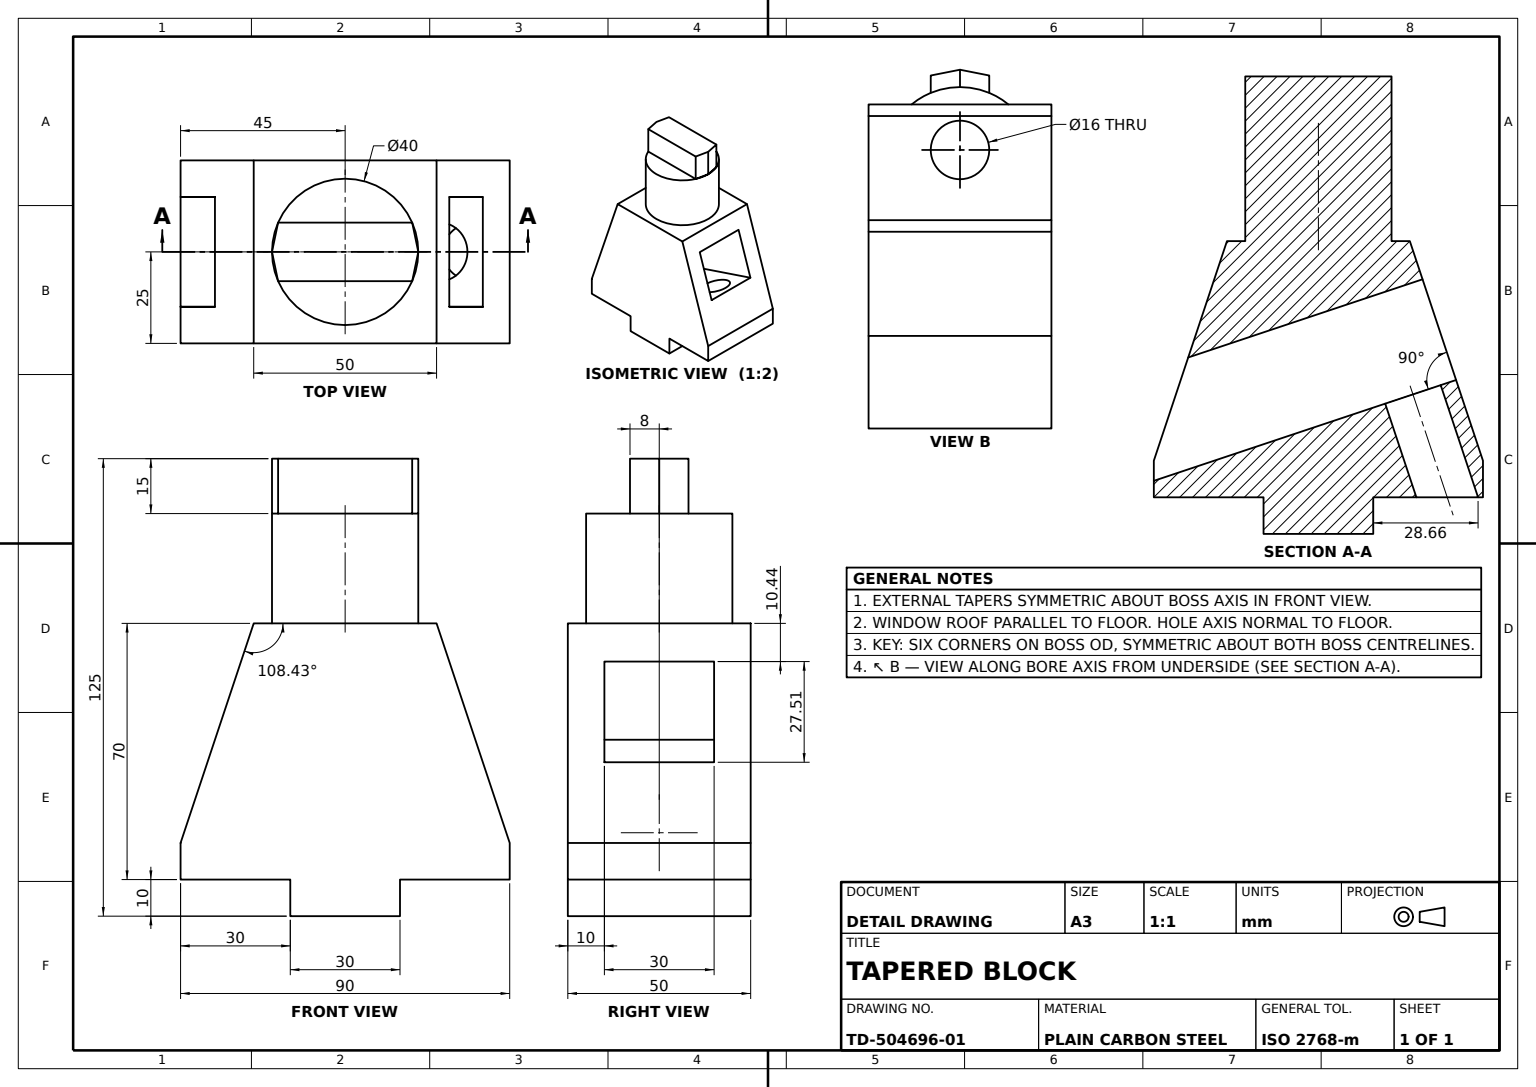
from build123d import *

# Parameters (mm, degrees)
BASE_BODY_DEPTH              = 50
SIDE_WINDOW_SKETCH_W         = 30
SIDE_WINDOW_SKETCH_H         = 29
SIDE_WINDOW_CUT_DEPTH        = 107.395488626
CYLINDRICAL_BOSS_40_SKETCH_R = 20
CYLINDRICAL_BOSS_40_DEPTH    = 30
TOP_KEY_DEPTH                = 15
HOLE_16_SKETCH_R             = 8
HOLE_16_DEPTH                = 153.165355608


with BuildPart() as part:
    # Base Body Profile Sketch → Base Body (new body)
    with BuildSketch(Plane.XY):
        Polygon((0, 0), (30, 0), (30, -10), (60, -10), (60, 0), (90, 0), (90, 10), (70, 70), (20, 70), (0, 10), align=None)
    extrude(amount=-BASE_BODY_DEPTH)

    # Side Window Sketch → Side Window Cut (cut, through all)
    with BuildSketch(Plane(origin=(84, 28, 0), x_dir=(0, 0, -1), z_dir=(0.948683298050514, 0.31622776601683783, 0))):
        with Locations((25, 18.771887242)):
            Rectangle(SIDE_WINDOW_SKETCH_W, SIDE_WINDOW_SKETCH_H)
    extrude(amount=-SIDE_WINDOW_CUT_DEPTH, mode=Mode.SUBTRACT)

    # Cylindrical Boss Ø40 Sketch → Cylindrical Boss Ø40 (add)
    with BuildSketch(Plane(origin=(0, 70, 0), x_dir=(1, 0, 0), z_dir=(0, 1, 0))):
        with Locations(Location((45, 25, 0), (0, 0, 270))):
            Circle(CYLINDRICAL_BOSS_40_SKETCH_R)
    extrude(amount=CYLINDRICAL_BOSS_40_DEPTH)

    # Top Key Sketch → Top Key (add)
    with BuildSketch(Plane(origin=(0, 100, 0), x_dir=(1, 0, 0), z_dir=(0, 1, 0))):
        Polygon((25, 25), (26.66969722, 33), (63.33030278, 33), (65, 25), (63.33030278, 17), (26.66969722, 17), align=None)
    extrude(amount=TOP_KEY_DEPTH)

    # Hole Ø16 Sketch → Hole Ø16 (cut, through all)
    with BuildSketch(Plane(origin=(-1.350889359, 4.052668078, 0), x_dir=(0.9486832980505139, 0.31622776601683794, 0), z_dir=(-0.31622776601683794, 0.9486832980505139, 0))):
        with Locations(Location((76.109609582, 25, 0), (0, 0, 180))):
            Circle(HOLE_16_SKETCH_R)
    extrude(amount=-HOLE_16_DEPTH, mode=Mode.SUBTRACT)


solid = part.part
